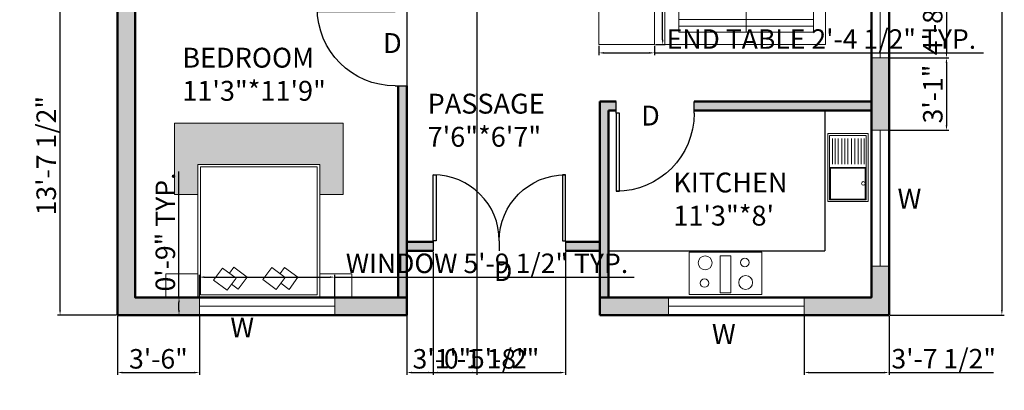
# Model space of a CAD drawing. Units: inches. Extents: x 1822 to 2392, y 2066 to 2908.
# Tile 1 of 4: x 1822 to 2328, y 2066 to 2256. Entities that reach past the tile are written whole.
import ezdxf

# ---------------------------------------------------------------- set-up
doc = ezdxf.new("R2010")
doc.units = ezdxf.units.IN
for name, color, linetype, lineweight in [('A-ANNO-DIMS', 2, 'Continuous', 18), ('A-AREA-IDEN', 83, 'Continuous', 25), ('A-FLOR-CASE', 132, 'Continuous', 25), ('A-FLOR-PATT', 9, 'Continuous', 13), ('A-FURN', 140, 'Continuous', 18), ('A-WALL-PATT', 252, 'Continuous', 13), ('BEDS', 40, 'Continuous', 18), ('DOOR', 50, 'Continuous', 25), ('KIT', 132, 'Continuous', 18), ('SOFA', 140, 'Continuous', 18), ('TEXT', 83, 'Continuous', 25), ('wall', 7, 'Continuous', 50), ('WINDOW', 80, 'Continuous', 20)]:
    doc.layers.add(name, color=color, linetype=linetype, lineweight=lineweight)
doc.styles.get("Standard").update_dxf_attribs({"font": 'arial.ttf'})
doc.dimstyles.new('ISO-25', dxfattribs={"dimtxt": 10, "dimasz": 2.5, "dimexe": 1.25, "dimexo": 0.625, "dimtad": 1, "dimdec": 0, "dimlunit": 4, "dimtxsty": 'Standard', "dimcen": 2.5, "dimadec": 0, "dimazin": 0, "dimtfac": 1, "dimtdec": 0, "dimtmove": 0, "dimatfit": 3, "dimfxl": 1, "dimarcsym": 0})

# ---------------------------------------------------------------- blocks, each defined once
blk = doc.blocks.new('*U2')
for p, q in [((0, 0), (0, -6)), ((40, 0), (40, -6))]:
    blk.add_line(p, q)
blk.add_lwpolyline([(0, 0), (0, 40), (1.75, 40), (1.75, 0)], close=True)
blk.add_arc((0, 0), 40, 0, 90)
blk = doc.blocks.new('*D6')
at = {"layer": 'A-ANNO-DIMS', "color": 0, "lineweight": -2, "transparency": 16777216}
for p, q in [((2269.04, 2584.12), (2327.59, 2584.12)), ((2326.34, 2581.62), (2326.34, 2106.62)), ((2269.04, 2104.12), (2327.59, 2104.12))]:
    blk.add_line(p, q, dxfattribs=at)
at = {"layer": 'A-ANNO-DIMS', "color": 0, "transparency": 16777216}
for points in [[(2325.93, 2581.62), (2326.76, 2581.62), (2326.34, 2584.12)], [(2325.93, 2106.62), (2326.76, 2106.62), (2326.34, 2104.12)]]:
    blk.add_solid(points, dxfattribs=at)
at = {"layer": 'Defpoints', "color": 0, "transparency": 16777216}
for p in [(2268.41, 2584.12), (2268.41, 2104.12), (2326.34, 2104.12)]:
    blk.add_point(p, dxfattribs=at)
at = {"layer": 'A-ANNO-DIMS', "color": 0, "transparency": 16777216, "insert": (2320.61, 2344.12), "char_height": 10, "attachment_point": 5, "rotation": 90}
blk.add_mtext("40'", dxfattribs=at)
blk = doc.blocks.new('BED-DOUBLE-WITH-NIGHTSTANDS')
for p, q in [((0, -52.84), (-12, -52.84)), ((-12, -52.84), (-12, -89.47)), ((62.55, -52.84), (74.55, -52.84)), ((74.55, -52.84), (74.55, -89.47)), ((-12, -89.47), (74.55, -89.47))]:
    blk.add_line(p, q)
for points in [[(0, 0), (-16.5, 0), (-16.5, -12.19), (0, -12.19)], [(0, 0), (62.55, 0), (62.55, -68.27), (0, -68.27)], [(79.04, 0), (62.55, 0), (62.55, -12.19), (79.04, -12.19)], [(1.28, -1.28), (61.27, -1.28), (61.27, -67), (1.28, -67)], [(22.38, -4.1), (29.25, -9.19), (24.65, -15.4), (17.78, -10.31)], [(47.61, -3.78), (54.48, -8.87), (49.87, -15.08), (43, -9.99)]]:
    blk.add_lwpolyline(points, close=True)
for points in [[(20.42, -12.27), (18.06, -15.45), (11.2, -10.36), (15.8, -4.15), (20.02, -7.28)], [(46.41, -12.52), (44.19, -15.51), (37.32, -10.42), (41.93, -4.21), (45.39, -6.77)]]:
    blk.add_lwpolyline(points)
blk = doc.blocks.new('SOFA-TWO-SEAT')
for p, q in [((0, 0), (0, 35.2)), ((0, 35.2), (82.54, 35.2)), ((82.54, 35.2), (82.54, 0)), ((7.18, 25.83), (76.33, 25.83)), ((41.75, 28.9), (41.75, 0)), ((7.18, 22.51), (76.33, 22.51)), ((7.18, 0), (0, 0)), ((82.54, 0), (73.14, 0))]:
    blk.add_line(p, q)
blk.add_lwpolyline([(76.33, 0), (7.18, 0), (7.18, 28.9), (76.33, 28.9)], close=True)
blk = doc.blocks.new('WINDOW-EXT-TYPE-A')
blk.add_line((0, 4.5), (69.61, 4.5))
blk.add_lwpolyline([(0, 9), (69.61, 9), (69.61, 0), (0, 0)], close=True)
blk = doc.blocks.new('TABLE-END')
blk.add_lwpolyline([(0, 0), (28.42, 0), (28.42, 23.78), (0, 23.78)], close=True)
blk = doc.blocks.new('*D14')
at = {"layer": 'A-ANNO-DIMS', "color": 0, "lineweight": -2, "transparency": 16777216}
for p, q in [((1914.42, 2113.74), (1914.42, 2124.81)), ((1916.92, 2123.56), (1981.53, 2123.56)), ((1984.03, 2113.74), (1984.03, 2124.81)), ((1984.03, 2123.56), (2137.62, 2123.56))]:
    blk.add_line(p, q, dxfattribs=at)
at = {"layer": 'A-ANNO-DIMS', "color": 0, "transparency": 16777216}
for points in [[(1916.92, 2123.97), (1916.92, 2123.14), (1914.42, 2123.56)], [(1981.53, 2123.97), (1981.53, 2123.14), (1984.03, 2123.56)]]:
    blk.add_solid(points, dxfattribs=at)
at = {"layer": 'Defpoints', "color": 0, "transparency": 16777216}
for p in [(1984.03, 2123.56), (1914.42, 2113.12), (1984.03, 2113.12)]:
    blk.add_point(p, dxfattribs=at)
at = {"layer": 'A-ANNO-DIMS', "color": 0, "transparency": 16777216, "insert": (2062.07, 2129.36), "char_height": 10, "attachment_point": 5}
blk.add_mtext('WINDOW 5\'-9 1/2" TYP.', dxfattribs=at)
blk = doc.blocks.new('*D15')
at = {"layer": 'A-ANNO-DIMS', "color": 0, "lineweight": -2, "transparency": 16777216}
for p, q in [((1903.97, 2113.12), (1903.97, 2177.82)), ((1913.79, 2113.12), (1902.72, 2113.12)), ((1903.97, 2106.62), (1903.97, 2110.62)), ((1913.79, 2104.12), (1902.72, 2104.12))]:
    blk.add_line(p, q, dxfattribs=at)
at = {"layer": 'A-ANNO-DIMS', "color": 0, "transparency": 16777216}
for points in [[(1903.56, 2110.62), (1904.39, 2110.62), (1903.97, 2113.12)], [(1903.56, 2106.62), (1904.39, 2106.62), (1903.97, 2104.12)]]:
    blk.add_solid(points, dxfattribs=at)
at = {"layer": 'Defpoints', "color": 0, "transparency": 16777216}
for p in [(1903.97, 2113.12), (1914.42, 2113.12), (1914.42, 2104.12)]:
    blk.add_point(p, dxfattribs=at)
at = {"layer": 'A-ANNO-DIMS', "color": 0, "transparency": 16777216, "insert": (1898.24, 2146.72), "char_height": 10, "attachment_point": 5, "rotation": 90}
blk.add_mtext('0\'-9" TYP.', dxfattribs=at)
blk = doc.blocks.new('*D24')
at = {"layer": 'A-ANNO-DIMS', "color": 0, "lineweight": -2, "transparency": 16777216}
for p, q in [((2119.55, 2242.25), (2119.55, 2237.36)), ((2147.97, 2242.25), (2147.97, 2237.36)), ((2122.05, 2238.61), (2145.47, 2238.61)), ((2147.97, 2238.61), (2316.96, 2238.61))]:
    blk.add_line(p, q, dxfattribs=at)
at = {"layer": 'A-ANNO-DIMS', "color": 0, "transparency": 16777216}
for points in [[(2122.05, 2239.03), (2122.05, 2238.2), (2119.55, 2238.61)], [(2145.47, 2239.03), (2145.47, 2238.2), (2147.97, 2238.61)]]:
    blk.add_solid(points, dxfattribs=at)
at = {"layer": 'Defpoints', "color": 0, "transparency": 16777216}
for p in [(2119.55, 2242.88), (2147.97, 2242.88), (2147.97, 2238.61)]:
    blk.add_point(p, dxfattribs=at)
at = {"layer": 'A-ANNO-DIMS', "color": 0, "transparency": 16777216, "insert": (2233.72, 2244.41), "char_height": 10, "attachment_point": 5}
blk.add_mtext('END TABLE 2\'-4 1/2" TYP.', dxfattribs=at)
blk = doc.blocks.new('*D25')
at = {"layer": 'A-ANNO-DIMS', "color": 0, "lineweight": -2, "transparency": 16777216}
for p, q in [((2152.23, 2266.66), (2152.23, 2331.53)), ((2148.59, 2266.66), (2153.48, 2266.66)), ((2152.23, 2245.38), (2152.23, 2264.16)), ((2148.59, 2242.88), (2153.48, 2242.88))]:
    blk.add_line(p, q, dxfattribs=at)
at = {"layer": 'A-ANNO-DIMS', "color": 0, "transparency": 16777216}
for points in [[(2151.81, 2264.16), (2152.65, 2264.16), (2152.23, 2266.66)], [(2151.81, 2245.38), (2152.65, 2245.38), (2152.23, 2242.88)]]:
    blk.add_solid(points, dxfattribs=at)
at = {"layer": 'Defpoints', "color": 0, "transparency": 16777216}
for p in [(2147.97, 2266.66), (2152.23, 2266.66), (2147.97, 2242.88)]:
    blk.add_point(p, dxfattribs=at)
at = {"layer": 'A-ANNO-DIMS', "color": 0, "transparency": 16777216, "insert": (2146.5, 2300.35), "char_height": 10, "attachment_point": 5, "rotation": 90}
blk.add_mtext('2\'-0" TYP.', dxfattribs=at)
blk = doc.blocks.new('*D35')
at = {"layer": 'A-ANNO-DIMS', "color": 0, "lineweight": -2, "transparency": 16777216}
for p, q in [((2269.04, 2292.4), (2299.16, 2292.4)), ((2297.91, 2289.9), (2297.91, 2238.6)), ((2269.04, 2236.1), (2299.16, 2236.1))]:
    blk.add_line(p, q, dxfattribs=at)
at = {"layer": 'A-ANNO-DIMS', "color": 0, "transparency": 16777216}
for points in [[(2297.5, 2289.9), (2298.33, 2289.9), (2297.91, 2292.4)], [(2297.5, 2238.6), (2298.33, 2238.6), (2297.91, 2236.1)]]:
    blk.add_solid(points, dxfattribs=at)
at = {"layer": 'Defpoints', "color": 0, "transparency": 16777216}
for p in [(2268.41, 2292.4), (2268.41, 2236.1), (2297.91, 2236.1)]:
    blk.add_point(p, dxfattribs=at)
at = {"layer": 'A-ANNO-DIMS', "color": 0, "transparency": 16777216, "insert": (2292.12, 2264.25), "char_height": 10, "attachment_point": 5, "rotation": 90}
blk.add_mtext('4\'-8 1/2"', dxfattribs=at)
blk = doc.blocks.new('*D36')
at = {"layer": 'A-ANNO-DIMS', "color": 0, "lineweight": -2, "transparency": 16777216}
for p, q in [((2269.04, 2236.1), (2299.16, 2236.1)), ((2297.91, 2233.6), (2297.91, 2201.38)), ((2269.04, 2198.88), (2299.16, 2198.88))]:
    blk.add_line(p, q, dxfattribs=at)
at = {"layer": 'A-ANNO-DIMS', "color": 0, "transparency": 16777216}
for points in [[(2297.5, 2233.6), (2298.33, 2233.6), (2297.91, 2236.1)], [(2297.5, 2201.38), (2298.33, 2201.38), (2297.91, 2198.88)]]:
    blk.add_solid(points, dxfattribs=at)
at = {"layer": 'Defpoints', "color": 0, "transparency": 16777216}
for p in [(2268.41, 2236.1), (2268.41, 2198.88), (2297.91, 2198.88)]:
    blk.add_point(p, dxfattribs=at)
at = {"layer": 'A-ANNO-DIMS', "color": 0, "transparency": 16777216, "insert": (2292.18, 2217.49), "char_height": 10, "attachment_point": 5, "rotation": 90}
blk.add_mtext('3\'-1"', dxfattribs=at)
blk = doc.blocks.new('*D37')
at = {"layer": 'A-ANNO-DIMS', "color": 0, "lineweight": -2, "transparency": 16777216}
for p, q in [((1872.41, 2103.49), (1872.41, 2073.37)), ((1914.42, 2103.49), (1914.42, 2073.37)), ((1874.91, 2074.62), (1911.92, 2074.62))]:
    blk.add_line(p, q, dxfattribs=at)
at = {"layer": 'A-ANNO-DIMS', "color": 0, "transparency": 16777216}
for points in [[(1874.91, 2075.03), (1874.91, 2074.2), (1872.41, 2074.62)], [(1911.92, 2075.03), (1911.92, 2074.2), (1914.42, 2074.62)]]:
    blk.add_solid(points, dxfattribs=at)
at = {"layer": 'Defpoints', "color": 0, "transparency": 16777216}
for p in [(1872.41, 2104.12), (1914.42, 2104.12), (1914.42, 2074.62)]:
    blk.add_point(p, dxfattribs=at)
at = {"layer": 'A-ANNO-DIMS', "color": 0, "transparency": 16777216, "insert": (1893.41, 2080.35), "char_height": 10, "attachment_point": 5}
blk.add_mtext('3\'-6"', dxfattribs=at)
blk = doc.blocks.new('*D38')
at = {"layer": 'A-ANNO-DIMS', "color": 0, "lineweight": -2, "transparency": 16777216}
for p, q in [((2224.8, 2103.49), (2224.8, 2073.37)), ((2268.41, 2103.49), (2268.41, 2073.37)), ((2227.3, 2074.62), (2265.91, 2074.62)), ((2268.41, 2074.62), (2322.04, 2074.62))]:
    blk.add_line(p, q, dxfattribs=at)
at = {"layer": 'A-ANNO-DIMS', "color": 0, "transparency": 16777216}
for points in [[(2227.3, 2075.03), (2227.3, 2074.2), (2224.8, 2074.62)], [(2265.91, 2075.03), (2265.91, 2074.2), (2268.41, 2074.62)]]:
    blk.add_solid(points, dxfattribs=at)
at = {"layer": 'Defpoints', "color": 0, "transparency": 16777216}
for p in [(2224.8, 2104.12), (2268.41, 2104.12), (2268.41, 2074.62)]:
    blk.add_point(p, dxfattribs=at)
at = {"layer": 'A-ANNO-DIMS', "color": 0, "transparency": 16777216, "insert": (2296.48, 2080.42), "char_height": 10, "attachment_point": 5}
blk.add_mtext('3\'-7 1/2"', dxfattribs=at)
blk = doc.blocks.new('*D41')
at = {"layer": 'A-ANNO-DIMS', "color": 0, "lineweight": -2, "transparency": 16777216}
for p, q in [((2020.91, 2488.49), (2020.91, 2073.37)), ((2056.91, 2488.49), (2056.91, 2073.37)), ((2023.41, 2074.62), (2054.41, 2074.62))]:
    blk.add_line(p, q, dxfattribs=at)
at = {"layer": 'A-ANNO-DIMS', "color": 0, "transparency": 16777216}
for points in [[(2023.41, 2075.03), (2023.41, 2074.2), (2020.91, 2074.62)], [(2054.41, 2075.03), (2054.41, 2074.2), (2056.91, 2074.62)]]:
    blk.add_solid(points, dxfattribs=at)
at = {"layer": 'Defpoints', "color": 0, "transparency": 16777216}
for p in [(2020.91, 2489.12), (2056.91, 2489.12), (2056.91, 2074.62)]:
    blk.add_point(p, dxfattribs=at)
at = {"layer": 'A-ANNO-DIMS', "color": 0, "transparency": 16777216, "insert": (2038.91, 2080.35), "char_height": 10, "attachment_point": 5}
blk.add_mtext('3\'-0"', dxfattribs=at)
blk = doc.blocks.new('*D42')
at = {"layer": 'A-ANNO-DIMS', "color": 0, "lineweight": -2, "transparency": 16777216}
for p, q in [((2034.48, 2136.49), (2034.48, 2073.37)), ((2102.28, 2136.49), (2102.28, 2073.37)), ((2036.98, 2074.62), (2099.78, 2074.62))]:
    blk.add_line(p, q, dxfattribs=at)
at = {"layer": 'A-ANNO-DIMS', "color": 0, "transparency": 16777216}
for points in [[(2036.98, 2075.03), (2036.98, 2074.2), (2034.48, 2074.62)], [(2099.78, 2075.03), (2099.78, 2074.2), (2102.28, 2074.62)]]:
    blk.add_solid(points, dxfattribs=at)
at = {"layer": 'Defpoints', "color": 0, "transparency": 16777216}
for p in [(2034.48, 2137.12), (2102.28, 2137.12), (2102.28, 2074.62)]:
    blk.add_point(p, dxfattribs=at)
at = {"layer": 'A-ANNO-DIMS', "color": 0, "transparency": 16777216, "insert": (2068.38, 2080.35), "char_height": 10, "attachment_point": 5}
blk.add_mtext('5\'-8"', dxfattribs=at)
blk = doc.blocks.new('*D45')
at = {"layer": 'A-ANNO-DIMS', "color": 0, "lineweight": -2, "transparency": 16777216}
for p, q in [((2020.91, 2136.49), (2020.91, 2073.37)), ((2034.48, 2136.49), (2034.48, 2073.37)), ((2023.41, 2074.62), (2031.98, 2074.62)), ((2034.48, 2074.62), (2087.17, 2074.62))]:
    blk.add_line(p, q, dxfattribs=at)
at = {"layer": 'A-ANNO-DIMS', "color": 0, "transparency": 16777216}
for points in [[(2023.41, 2075.03), (2023.41, 2074.2), (2020.91, 2074.62)], [(2031.98, 2075.03), (2031.98, 2074.2), (2034.48, 2074.62)]]:
    blk.add_solid(points, dxfattribs=at)
at = {"layer": 'Defpoints', "color": 0, "transparency": 16777216}
for p in [(2020.91, 2137.12), (2034.48, 2137.12), (2034.48, 2074.62)]:
    blk.add_point(p, dxfattribs=at)
at = {"layer": 'A-ANNO-DIMS', "color": 0, "transparency": 16777216, "insert": (2062.08, 2080.41), "char_height": 10, "attachment_point": 5}
blk.add_mtext('1\'-1 1/2"', dxfattribs=at)
blk = doc.blocks.new('*D46')
at = {"layer": 'A-ANNO-DIMS', "color": 0, "lineweight": -2, "transparency": 16777216}
for p, q in [((1880.79, 2267.62), (1841.66, 2267.62)), ((1842.91, 2106.62), (1842.91, 2265.12)), ((1871.79, 2104.12), (1841.66, 2104.12))]:
    blk.add_line(p, q, dxfattribs=at)
at = {"layer": 'A-ANNO-DIMS', "color": 0, "transparency": 16777216}
for points in [[(1842.5, 2265.12), (1843.33, 2265.12), (1842.91, 2267.62)], [(1842.5, 2106.62), (1843.33, 2106.62), (1842.91, 2104.12)]]:
    blk.add_solid(points, dxfattribs=at)
at = {"layer": 'Defpoints', "color": 0, "transparency": 16777216}
for p in [(1842.91, 2267.62), (1881.41, 2267.62), (1872.41, 2104.12)]:
    blk.add_point(p, dxfattribs=at)
at = {"layer": 'A-ANNO-DIMS', "color": 0, "transparency": 16777216, "insert": (1837.11, 2185.87), "char_height": 10, "attachment_point": 5, "rotation": 90}
blk.add_mtext('13\'-7 1/2"', dxfattribs=at)

msp = doc.modelspace()

# ---------------------------------------------------------------- hatches: boundary and pattern name
at = {"layer": 'A-FLOR-PATT'}
h = msp.add_hatch(dxfattribs=at)
h.set_pattern_fill('ANSI36', color=256)
h.paths.add_polyline_path([(1983.57, 2522.27), (1971.57, 2522.27), (1971.57, 2506.84), (1909.02, 2506.84), (1909.02, 2522.27), (1897.02, 2522.27), (1897.02, 2485.65), (1983.57, 2485.65)])
h.paths.add_polyline_path([(1988.24, 2202.59), (1901.7, 2202.59), (1901.7, 2165.96), (1913.7, 2165.96), (1913.7, 2181.39), (1976.24, 2181.39), (1976.24, 2165.96), (1988.24, 2165.96)])
h.paths.add_polyline_path([(2250.08, 2522.27), (2238.08, 2522.27), (2238.08, 2506.84), (2175.53, 2506.84), (2175.53, 2522.27), (2163.53, 2522.27), (2163.53, 2485.65), (2250.08, 2485.65)])
at = {"layer": 'A-WALL-PATT'}
h = msp.add_hatch(color=256, dxfattribs=at)
h.dxf.hatch_style = 1
h.paths.add_polyline_path([(2032.62, 2584.12), (1982.01, 2584.12), (1982.01, 2575.12), (1988.06, 2575.12), (2016.41, 2575.12), (2032.62, 2575.12)], flags=17)
h.paths.add_polyline_path([(2156.61, 2584.12), (2102.23, 2584.12), (2102.23, 2575.12), (2119.91, 2575.12), (2156.61, 2575.12)], flags=17)
h.paths.add_polyline_path([(1914.42, 2104.12), (1914.42, 2113.12), (1881.41, 2113.12), (1881.41, 2575.12), (1912.4, 2575.12), (1912.4, 2584.12), (1872.41, 2584.12), (1872.41, 2104.12)])
h.paths.add_polyline_path([(2268.41, 2129.27), (2259.41, 2129.27), (2259.41, 2113.12), (2224.8, 2113.12), (2224.8, 2104.12), (2268.41, 2104.12)])
h.paths.add_polyline_path([(2268.41, 2236.1), (2259.41, 2236.1), (2259.41, 2198.88), (2268.41, 2198.88)])
h.paths.add_polyline_path([(2268.41, 2358.32), (2259.41, 2358.32), (2259.41, 2292.4), (2268.41, 2292.4)])
h.paths.add_polyline_path([(2259.41, 2554.73), (2268.41, 2554.73), (2268.41, 2584.12), (2226.22, 2584.12), (2226.22, 2575.12), (2259.41, 2575.12)])
h.paths.add_polyline_path([(2268.41, 2485.12), (2259.41, 2485.12), (2259.41, 2408.76), (2268.41, 2408.76)])
h.paths.add_polyline_path([(2020.91, 2104.12), (2020.91, 2113.12), (1984.03, 2113.12), (1984.03, 2104.12)])
h.paths.add_polyline_path([(2119.91, 2113.12), (2119.91, 2104.12), (2155.19, 2104.12), (2155.19, 2113.12)])
h = msp.add_hatch(color=256, dxfattribs=at)
h.dxf.hatch_style = 1
h.paths.add_polyline_path([(2124.41, 2575.12), (2119.91, 2575.12), (2119.91, 2471.52), (2124.41, 2471.52)])
h.paths.add_polyline_path([(2020.91, 2575.12), (2016.41, 2575.12), (2016.41, 2471.18), (2020.91, 2471.18)])
h.paths.add_polyline_path([(2259.41, 2428.12), (2124.41, 2428.12), (2124.41, 2431.52), (2119.91, 2431.52), (2119.91, 2423.62), (2259.41, 2423.62)])
h.paths.add_polyline_path([(2020.91, 2363.62), (2016.41, 2363.62), (2015.38, 2363.62), (2015.38, 2359.12), (2016.41, 2359.12), (2016.41, 2272.12), (1945.91, 2272.12), (1945.91, 2305.88), (1941.41, 2305.88), (1941.41, 2272.12), (1923.14, 2272.12), (1923.14, 2267.62), (2016.41, 2267.62), (2016.41, 2261.67), (2020.91, 2261.67), (2020.91, 2267.62)])
h.paths.add_polyline_path([(2259.41, 2213.62), (2168.4, 2213.62), (2168.4, 2209.12), (2259.41, 2209.12)])
h.paths.add_polyline_path([(2124.41, 2209.12), (2128.4, 2209.12), (2128.4, 2213.62), (2119.91, 2213.62), (2119.91, 2113.12), (2124.41, 2113.12), (2124.41, 2137.12)])
h.paths.add_polyline_path([(2020.91, 2221.67), (2016.41, 2221.67), (2016.41, 2113.12), (2020.91, 2113.12), (2020.91, 2137.12)])
h.paths.add_polyline_path([(2034.48, 2141.62), (2020.91, 2141.62), (2020.91, 2137.12), (2034.48, 2137.12)])
h.paths.add_polyline_path([(2119.91, 2141.62), (2102.28, 2141.62), (2102.28, 2137.12), (2119.91, 2137.12)])
h.paths.add_polyline_path([(1973.91, 2423.62), (1969.41, 2423.62), (1969.41, 2399.09), (1973.91, 2399.09)])

# ---------------------------------------------------------------- linework, layer by layer
at = {"layer": 'A-FLOR-CASE'}
for p, q in [((2259.41, 2209.12), (2235.41, 2209.12)), ((2235.41, 2209.12), (2235.41, 2137.12)), ((2124.41, 2113.12), (2124.41, 2137.12)), ((2124.41, 2137.12), (2235.41, 2137.12))]:
    msp.add_line(p, q, dxfattribs=at)
at = {"layer": 'KIT'}
for p, q in [((2239.44, 2194.71), (2239.44, 2181.6)), ((2240.81, 2194.71), (2240.81, 2181.6)), ((2242.4, 2194.71), (2242.4, 2181.6)), ((2244.14, 2194.71), (2244.14, 2181.6)), ((2245.73, 2194.71), (2245.73, 2181.6)), ((2247.31, 2194.71), (2247.31, 2181.6)), ((2249.17, 2194.71), (2249.17, 2181.6)), ((2250.81, 2194.71), (2250.81, 2181.6)), ((2252.51, 2194.71), (2252.51, 2181.6)), ((2254.09, 2194.71), (2254.09, 2181.6)), ((2255.62, 2194.71), (2255.62, 2181.6)), ((2237.95, 2179.78), (2256.72, 2179.78))]:
    msp.add_line(p, q, dxfattribs=at)
for points in [[(2236.95, 2197.27), (2257.72, 2197.27), (2257.72, 2162.3), (2236.95, 2162.3)], [(2237.95, 2196.27), (2256.72, 2196.27), (2256.72, 2163.3), (2237.95, 2163.3)], [(2238.35, 2179.53), (2256.23, 2179.53), (2256.23, 2163.58), (2238.35, 2163.58)], [(2165.88, 2114.65), (2203.18, 2114.65), (2203.18, 2136.34), (2165.88, 2136.34)], [(2181.82, 2134.51), (2187.25, 2134.51), (2187.25, 2115.58), (2181.82, 2115.58)]]:
    msp.add_lwpolyline(points, close=True, dxfattribs=at)
for centre, radius in [((2255.21, 2171.64), 0.928), ((2174.09, 2130.89), 3.57), ((2194.39, 2131.06), 2.19), ((2173.74, 2120.53), 2.19), ((2194.82, 2120.79), 3.57)]:
    msp.add_circle(centre, radius, dxfattribs=at)
at = {"layer": 'wall'}
for p, q in [((1881.41, 2267.62), (1881.41, 2126.62)), ((2016.41, 2221.67), (2016.41, 2113.12)), ((2020.91, 2221.67), (2020.91, 2113.12)), ((2119.91, 2213.62), (2128.4, 2213.62)), ((2119.91, 2113.12), (2119.91, 2213.62)), ((2124.41, 2113.12), (2124.41, 2209.12)), ((2124.41, 2209.12), (2128.4, 2209.12)), ((2168.4, 2213.62), (2259.41, 2213.62)), ((2168.4, 2209.12), (2259.41, 2209.12)), ((2020.91, 2141.62), (2034.48, 2141.62)), ((2102.28, 2141.62), (2119.91, 2141.62)), ((2020.91, 2113.12), (2020.91, 2137.12)), ((2020.91, 2137.12), (2034.48, 2137.12)), ((2102.28, 2137.12), (2119.91, 2137.12)), ((2020.91, 2113.12), (2020.91, 2104.12)), ((2119.91, 2113.12), (2119.91, 2104.12)), ((2259.41, 2113.12), (2124.41, 2113.12))]:
    msp.add_line(p, q, dxfattribs=at)
for points in [[(2119.91, 2104.12), (2268.41, 2104.12), (2268.41, 2584.12), (1872.41, 2584.12), (1872.41, 2104.12), (2020.91, 2104.12)], [(2119.91, 2113.12), (2259.41, 2113.12), (2259.41, 2575.12), (1881.41, 2575.12), (1881.41, 2113.12), (2020.91, 2113.12)]]:
    msp.add_lwpolyline(points, dxfattribs=at)
at = {"layer": 'WINDOW'}
msp.add_line((2263.91, 2292.4), (2263.91, 2236.1), dxfattribs=at)
msp.add_lwpolyline([(2268.41, 2292.4), (2268.41, 2236.1), (2259.41, 2236.1), (2259.41, 2292.4)], close=True, dxfattribs=at)

# ---------------------------------------------------------------- block references
at = {"layer": 'A-FURN'}
msp.add_blockref('TABLE-END', (2119.55, 2242.88), dxfattribs=at)
at = {"layer": 'BEDS', "rotation": 180}
msp.add_blockref('BED-DOUBLE-WITH-NIGHTSTANDS', (1976.24, 2113.12), dxfattribs=at)
at = {"layer": 'DOOR', "xscale": -1}
for p, rotation in [((2014.91, 2261.67), 90), ((2128.4, 2207.62), 180)]:
    msp.add_blockref('*U2', p, dxfattribs=dict(at, rotation=rotation))
at = {"layer": 'DOOR', "yscale": 0.8475605218727595, "zscale": 0.8475605218727595}
for p, xscale in [((2034.48, 2142.2), 0.8475605218727595), ((2102.28, 2142.2), -0.8475605218727595)]:
    msp.add_blockref('*U2', p, dxfattribs=dict(at, xscale=xscale))
at = {"layer": 'SOFA', "extrusion": (0, 0, -1), "zscale": -1, "rotation": 180}
msp.add_blockref('SOFA-TWO-SEAT', (-2153.31, 2278.17), dxfattribs=at)
at = {"layer": 'WINDOW', "rotation": 269.9999999999973}
msp.add_blockref('WINDOW-EXT-TYPE-A', (2259.41, 2198.88), dxfattribs=at)
at = {"layer": 'WINDOW'}
for p in [(1914.42, 2104.12), (2155.19, 2104.12)]:
    msp.add_blockref('WINDOW-EXT-TYPE-A', p, dxfattribs=at)

# ---------------------------------------------------------------- texts
at = {"layer": 'A-AREA-IDEN', "attachment_point": 1}
for s, insert, char_height in [('BEDROOM\\P11\'3"*11\'9"', (1905.66, 2241.24), 10.1937), ('PASSAGE\\P7\'6"*6\'7"', (2031.6, 2217.65), 10.194), ('KITCHEN\\P11\'3"*8\'', (2157.71, 2177.2), 10.194)]:
    msp.add_mtext_dynamic_manual_height_columns(s, width=251.9343, gutter_width=50.97, heights=[0], dxfattribs=dict(at, insert=insert, char_height=char_height))
at = {"layer": 'TEXT', "char_height": 10.19, "attachment_point": 1}
for s, insert in [('D', (2008.73, 2248.75)), ('D', (2141.2, 2211.52)), ('W', (2272.8, 2168.9)), ('D', (2065.54, 2131.74)), ('W', (1930.31, 2102.83)), ('W', (2177.51, 2099.45))]:
    msp.add_mtext_dynamic_manual_height_columns(s, width=251.9343, gutter_width=50.97, heights=[0], dxfattribs=dict(at, insert=insert))

# ---------------------------------------------------------------- dimensions: what is measured, and where the dimension line sits
at = {"layer": 'A-ANNO-DIMS'}
for base, p1, p2, override, picture, middle in [((2326.34, 2104.12), (2268.41, 2584.12), (2268.41, 2104.12), {"dimclrd": 0, "dimclre": 0, "dimclrt": 0}, '*D6', (2320.61, 2344.12)), ((2297.91, 2236.1), (2268.41, 2292.4), (2268.41, 2236.1), {"dimdec": 1, "dimlfac": 1, "dimrnd": 0, "dimzin": 1, "dimdsep": 46, "dimlunit": 4, "dimfrac": 2}, '*D35', (2292.12, 2264.25)), ((1842.91, 2267.62), (1872.41, 2104.12), (1881.41, 2267.62), {"dimdec": 1, "dimlfac": 1, "dimrnd": 0, "dimzin": 1, "dimdsep": 46, "dimlunit": 4, "dimfrac": 2}, '*D46', (1837.11, 2185.87)), ((2297.91, 2198.88), (2268.41, 2236.1), (2268.41, 2198.88), {"dimdec": 1, "dimlfac": 1, "dimrnd": 0, "dimzin": 1, "dimdsep": 46, "dimlunit": 4, "dimfrac": 2}, '*D36', (2292.18, 2217.49))]:
    dim = msp.add_linear_dim(base=base, p1=p1, p2=p2, angle=90, dimstyle='ISO-25', override=override, dxfattribs=at)
    dim.commit()
    dim.dimension.update_dxf_attribs({"geometry": picture, "text_midpoint": middle})
for base, p1, p2, picture, middle in [((2056.91, 2074.62), (2020.91, 2489.12), (2056.91, 2489.12), '*D41', (2038.91, 2080.35)), ((2034.48, 2074.62), (2020.91, 2137.12), (2034.48, 2137.12), '*D45', (2062.08, 2080.41)), ((2102.28, 2074.62), (2034.48, 2137.12), (2102.28, 2137.12), '*D42', (2068.38, 2080.35)), ((1914.42, 2074.62), (1872.41, 2104.12), (1914.42, 2104.12), '*D37', (1893.41, 2080.35)), ((2268.41, 2074.62), (2224.8, 2104.12), (2268.41, 2104.12), '*D38', (2296.48, 2080.42))]:
    dim = msp.add_linear_dim(base=base, p1=p1, p2=p2, dimstyle='ISO-25', override={"dimdec": 1, "dimlfac": 1, "dimrnd": 0, "dimzin": 1, "dimdsep": 46, "dimlunit": 4, "dimfrac": 2}, dxfattribs=at)
    dim.commit()
    dim.dimension.update_dxf_attribs({"geometry": picture, "text_midpoint": middle})
for base, p1, p2, picture, middle in [((2152.23, 2266.66), (2147.97, 2242.88), (2147.97, 2266.66), '*D25', (2146.5, 2300.35)), ((1903.97, 2113.12), (1914.42, 2104.12), (1914.42, 2113.12), '*D15', (1898.24, 2146.72))]:
    dim = msp.add_linear_dim(base=base, p1=p1, p2=p2, angle=90, text='<> TYP.', dimstyle='ISO-25', override={"dimdec": 1, "dimlfac": 1, "dimrnd": 0, "dimzin": 1, "dimdsep": 46, "dimlunit": 4, "dimfrac": 2}, dxfattribs=at)
    dim.commit()
    dim.dimension.update_dxf_attribs({"geometry": picture, "text_midpoint": middle})
for base, p1, p2, text, picture, middle in [((2147.97, 2238.61), (2119.55, 2242.88), (2147.97, 2242.88), 'END TABLE <> TYP.', '*D24', (2233.72, 2244.41)), ((1984.03, 2123.56), (1914.42, 2113.12), (1984.03, 2113.12), 'WINDOW <> TYP.', '*D14', (2062.07, 2129.36))]:
    dim = msp.add_linear_dim(base=base, p1=p1, p2=p2, text=text, dimstyle='ISO-25', override={"dimdec": 1, "dimlfac": 1, "dimrnd": 0, "dimzin": 1, "dimdsep": 46, "dimlunit": 4, "dimfrac": 2}, dxfattribs=at)
    dim.commit()
    dim.dimension.update_dxf_attribs({"geometry": picture, "text_midpoint": middle})

doc.saveas('drawing.dxf')
